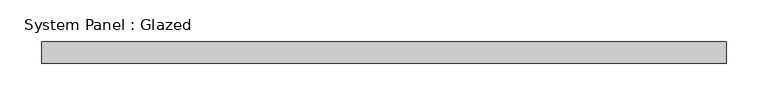
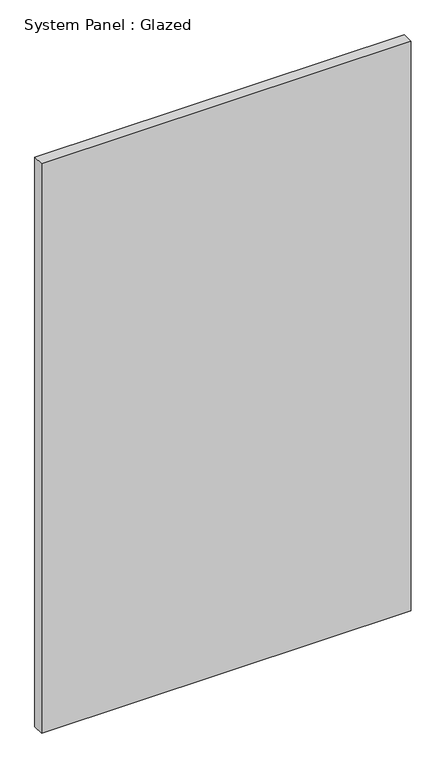
"""IFC4 building model written with IfcOpenShell, lengths in millimetres: plate geometry, System Panel : Glazed."""

from ifc_helpers import new_model, si_unit, origin, origin_with_axes, place, context, project, spatial, polyline, outline, extrude, source, transform, mapped, element, save


def system_panel_glazed_d91b2d6b(model_context):
    return source(origin(), model_context, "Body", "SweptSolid", [
        extrude(outline(polyline([(409.575, 19.05), (-409.575, 19.05), (-409.575, 44.45), (409.575, 44.45), (409.575, 19.05)])), origin_with_axes(), (0.0, 0.0, 1.0), 1332.9491558),
    ])


if __name__ == "__main__":
    model = new_model("IFC4")
    model_context = context("Model", 3, world=origin())
    ifc_project = project(units=[si_unit("LENGTHUNIT", "METRE", prefix="MILLI")], contexts=[model_context])
    site = spatial("IfcSite", under=ifc_project)
    building = spatial("IfcBuilding", under=site)
    placement = place(None, origin())
    system_panel_glazed_shape = system_panel_glazed_d91b2d6b(model_context)
    element("IfcPlate", 1, ObjectType="System Panel : Glazed", at=placement, inside=building, context=model_context, shape_type="MappedRepresentation", body=[
        mapped(system_panel_glazed_shape, transform((0.0, 0.0, 0.0), x_axis=(1.0, 0.0, 0.0), y_axis=(0.0, 1.0, 0.0), z_axis=(0.0, 0.0, 1.0))),
    ])
    save(model, "model.ifc")

# Revit data of these elements
# Type "System Panel : Glazed"
#   Construction Type Id = "GSP4R"
#   Analytic Construction = "1/8 in Pilkington single glazing"
#   Visual Light Transmittance = 0.9
#   Solar Heat Gain Coefficient = 0.86
#   Heat Transfer Coefficient (U) = 1.18115 BTU/(h·ft²·°F)
#   Define Thermal Properties by = 1
# Element 1 (IfcPlate, "System Panel : Glazed")
#   Materials on its faces: "Glass"
# Materials
#   "Glass": class "Glass", colour RGB 0 128 192, transparency 0.75, Description = "Soda Lime Glass", Cost = 0
